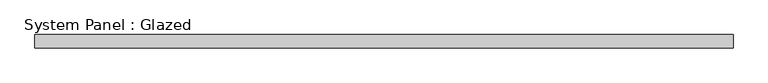
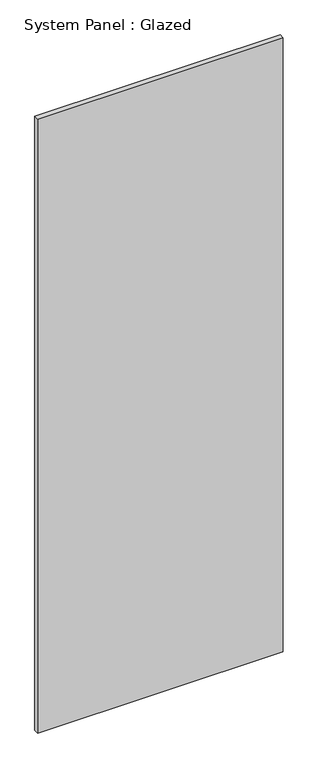
"""IFC4 building model written with IfcOpenShell, lengths in millimetres: plate geometry, System Panel : Glazed."""

from ifc_helpers import new_model, si_unit, origin, origin_with_axes, place, context, project, spatial, polyline, outline, extrude, source, transform, mapped, element, save


def system_panel_glazed_f24f7e4d(model_context):
    return source(origin(), model_context, "Body", "SweptSolid", [
        extrude(outline(polyline([(668.5577143, 19.05), (-668.5577143, 19.05), (-668.5577143, 44.45), (668.5577143, 44.45), (668.5577143, 19.05)])), origin_with_axes(), (0.0, 0.0, 1.0), 3530.6),
    ])


if __name__ == "__main__":
    model = new_model("IFC4")
    model_context = context("Model", 3, world=origin())
    ifc_project = project(units=[si_unit("LENGTHUNIT", "METRE", prefix="MILLI")], contexts=[model_context])
    site = spatial("IfcSite", under=ifc_project)
    building = spatial("IfcBuilding", under=site)
    placement = place(None, origin())
    system_panel_glazed_shape = system_panel_glazed_f24f7e4d(model_context)
    element("IfcPlate", 1, ObjectType="System Panel : Glazed", at=placement, inside=building, context=model_context, shape_type="MappedRepresentation", body=[
        mapped(system_panel_glazed_shape, transform((0.0, 0.0, 0.0), x_axis=(1.0, 0.0, 0.0), y_axis=(0.0, 1.0, 0.0), z_axis=(0.0, 0.0, 1.0))),
    ])
    save(model, "model.ifc")

# Revit data of these elements
# Type "System Panel : Glazed"
#   Construction Type Id = "GSP4R"
#   Analytic Construction = "1/8 in Pilkington single glazing"
#   Visual Light Transmittance = 0.9
#   Solar Heat Gain Coefficient = 0.86
#   Heat Transfer Coefficient (U) = 1.18115 BTU/(h·ft²·°F)
# Element 1 (IfcPlate, "System Panel : Glazed")
#   Materials on its faces: "Glass"
# Materials
#   "Glass": class "Glass", colour RGB 0 128 192, transparency 0.75, Description = "Soda Lime Glass", Cost = 0
